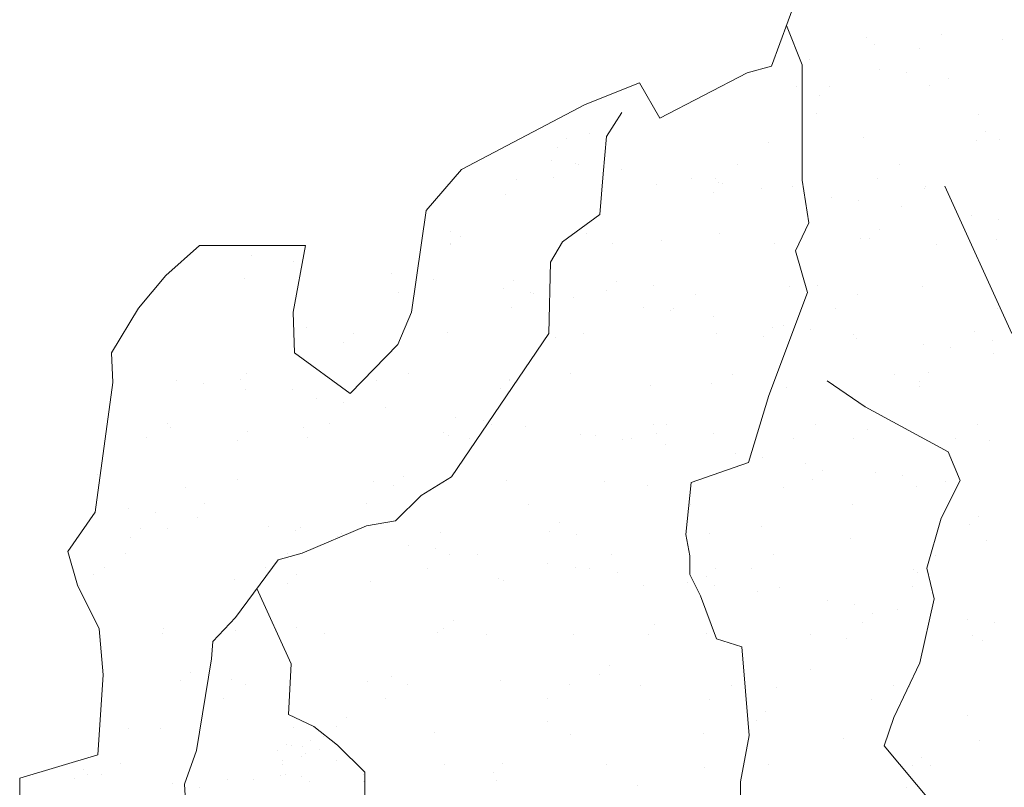
# Model space of a CAD drawing. Units: inches. Extents: x 1986 to 21484, y -1816 to 2016.
# Tile 19 of 85: x 2150.111 to 2157.681, y 1892.429 to 1898.331. Entities that reach past the tile are written whole.
import ezdxf

# ---------------------------------------------------------------- set-up
doc = ezdxf.new("R2010")
doc.units = ezdxf.units.IN
doc.layers.add('L-PLNT', color=84, linetype='Continuous', lineweight=13)

# ---------------------------------------------------------------- blocks, each defined once
blk = doc.blocks.new('PLANT-SHRUB')
for p, q in [((2155.8904, 1897.9733), (2156.12, 1898.5989)), ((2156.1272, 1897.9836), (2156.0052, 1898.2861)), ((2156.6216, 1898.1917), (2156.6216, 1898.1917)), ((2157.1978, 1898.2196), (2157.1978, 1898.2196)), ((2157.6678, 1898.1784), (2157.6678, 1898.1784)), ((2156.6845, 1898.1369), (2156.6845, 1898.1369)), ((2157.0293, 1898.1122), (2157.0293, 1898.1122)), ((2156.1795, 1898.0231), (2156.1795, 1898.0231)), ((2155.7025, 1897.9211), (2155.8904, 1897.9733)), ((2156.1272, 1897.7988), (2156.1272, 1897.9836)), ((2156.7223, 1897.9516), (2156.7223, 1897.9516)), ((2155.0321, 1897.574), (2155.7025, 1897.9211)), ((2156.9304, 1897.9242), (2156.9304, 1897.9242)), ((2157.2553, 1897.8814), (2157.2553, 1897.8814)), ((2154.4581, 1897.6783), (2154.8755, 1897.8452)), ((2154.8755, 1897.8452), (2155.0321, 1897.574)), ((2156.0812, 1897.817), (2156.0812, 1897.817)), ((2156.1275, 1897.0972), (2156.1272, 1897.7988)), ((2156.3368, 1897.8183), (2156.3368, 1897.8183)), ((2157.1035, 1897.8219), (2157.1035, 1897.8219)), ((2156.2632, 1897.7508), (2156.2632, 1897.7508)), ((2153.5085, 1897.1778), (2154.4581, 1897.6783)), ((2154.6228, 1897.4336), (2154.7404, 1897.6164)), ((2154.7404, 1897.6164), (2154.7404, 1897.6164)), ((2156.2372, 1897.6076), (2156.2372, 1897.6076)), ((2157.4818, 1897.6053), (2157.4818, 1897.6053)), ((2154.3162, 1897.4184), (2154.3162, 1897.4184)), ((2154.4945, 1897.4556), (2154.4945, 1897.4556)), ((2154.5967, 1897.1463), (2154.6228, 1897.4336)), ((2156.5964, 1897.4216), (2156.5964, 1897.4216)), ((2157.5383, 1897.4675), (2157.5383, 1897.4675)), ((2157.6426, 1897.4083), (2157.6426, 1897.4083)), ((2154.2425, 1897.3509), (2154.2425, 1897.3509)), ((2155.8654, 1897.3862), (2155.8654, 1897.3862)), ((2157.4646, 1897.4), (2157.4646, 1897.4)), ((2154.2022, 1897.2486), (2154.2022, 1897.2486)), ((2154.3858, 1897.2233), (2154.3858, 1897.2233)), ((2154.4102, 1897.2212), (2154.4102, 1897.2212)), ((2155.6304, 1897.2211), (2155.6304, 1897.2211)), ((2156.875, 1897.2188), (2156.875, 1897.2188)), ((2153.2371, 1896.865), (2153.5085, 1897.1778)), ((2154.2172, 1897.1159), (2154.2172, 1897.1159)), ((2154.5705, 1896.8329), (2154.5967, 1897.1463)), ((2154.7352, 1897.1784), (2154.7352, 1897.1784)), ((2155.278, 1897.1069), (2155.278, 1897.1069)), ((2155.4619, 1897.1137), (2155.4619, 1897.1137)), ((2156.7065, 1897.1114), (2156.7065, 1897.1114)), ((2153.9303, 1897.0992), (2153.9303, 1897.0992)), ((2155.0098, 1897.0603), (2155.0098, 1897.0603)), ((2155.4861, 1897.0795), (2155.4861, 1897.0795)), ((2155.5177, 1897.0676), (2155.5177, 1897.0676)), ((2155.811, 1897.0368), (2155.811, 1897.0368)), ((2156.056, 1897.0469), (2156.056, 1897.0469)), ((2156.1275, 1897.0972), (2156.1275, 1897.0972)), ((2156.1788, 1896.7685), (2156.1275, 1897.0972)), ((2157.0668, 1897.0355), (2157.0668, 1897.0355)), ((2157.0784, 1897.0518), (2157.0784, 1897.0518)), ((2157.224, 1897.0515), (2157.739, 1895.9176)), ((2153.8447, 1896.9864), (2153.8447, 1896.9864)), ((2155.444, 1897.0001), (2155.444, 1897.0001)), ((2156.3538, 1896.9653), (2156.3538, 1896.9653)), ((2156.5619, 1896.9379), (2156.5619, 1896.9379)), ((2156.8868, 1896.8951), (2156.8868, 1896.8951)), ((2153.1223, 1896.0829), (2153.2371, 1896.865)), ((2153.2371, 1896.865), (2153.2371, 1896.865)), ((2154.283, 1896.624), (2154.5705, 1896.8329)), ((2157.4297, 1896.8237), (2157.4297, 1896.8237)), ((2156.0761, 1896.5528), (2156.1788, 1896.7685)), ((2157.6377, 1896.7963), (2157.6377, 1896.7963)), ((2153.4232, 1896.6989), (2153.4232, 1896.6989)), ((2153.497, 1896.6678), (2153.497, 1896.6678)), ((2154.4694, 1896.6855), (2154.4694, 1896.6855)), ((2155.4918, 1896.6904), (2155.4918, 1896.6904)), ((2156.5712, 1896.6515), (2156.5712, 1896.6515)), ((2156.7191, 1896.7168), (2156.7191, 1896.7168)), ((2151.2335, 1896.3644), (2151.4944, 1896.5938)), ((2151.4944, 1896.5938), (2152.3084, 1896.5938)), ((2152.3084, 1896.5938), (2152.2144, 1896.0829)), ((2153.4233, 1896.6003), (2153.4233, 1896.6003)), ((2153.4251, 1896.6113), (2153.4251, 1896.6113)), ((2154.1915, 1896.4672), (2154.283, 1896.624)), ((2154.6697, 1896.609), (2154.6697, 1896.609)), ((2155.0462, 1896.6356), (2155.0462, 1896.6356)), ((2155.9144, 1896.6068), (2155.9144, 1896.6068)), ((2156.6455, 1896.6493), (2156.6455, 1896.6493)), ((2157.159, 1896.6045), (2157.159, 1896.6045)), ((2157.6174, 1896.6382), (2157.6174, 1896.6382)), ((2151.8901, 1896.5182), (2151.8901, 1896.5182)), ((2156.1686, 1896.2344), (2156.0761, 1896.5528)), ((2152.215, 1896.4754), (2152.215, 1896.4754)), ((2154.1785, 1895.9188), (2154.1915, 1896.4672)), ((2151.0248, 1896.1142), (2151.2335, 1896.3644)), ((2152.9659, 1896.3765), (2152.9659, 1896.3765)), ((2151.8366, 1896.3375), (2151.8366, 1896.3375)), ((2153.2908, 1896.3337), (2153.2908, 1896.3337)), ((2153.9052, 1896.3291), (2153.9052, 1896.3291)), ((2154.6985, 1896.317), (2154.6985, 1896.317)), ((2154.9846, 1896.2902), (2154.9846, 1896.2902)), ((2156.0308, 1896.2768), (2156.0308, 1896.2768)), ((2156.2476, 1896.2848), (2156.2476, 1896.2848)), ((2157.0532, 1896.2817), (2157.0532, 1896.2817)), ((2153.0255, 1896.2357), (2153.0255, 1896.2357)), ((2153.8337, 1896.2623), (2153.8337, 1896.2623)), ((2154.0417, 1896.2349), (2154.0417, 1896.2349)), ((2154.063, 1896.2225), (2154.063, 1896.2225)), ((2154.6248, 1896.2495), (2154.6248, 1896.2495)), ((2155.3076, 1896.2202), (2155.3076, 1896.2202)), ((2155.8693, 1895.4412), (2156.1686, 1896.2344)), ((2156.5523, 1896.218), (2156.5523, 1896.218)), ((2154.3667, 1896.1921), (2154.3667, 1896.1921)), ((2150.8161, 1895.7701), (2151.0248, 1896.1142)), ((2152.2144, 1896.0829), (2152.2249, 1895.7701)), ((2153.018, 1895.8326), (2153.1223, 1896.0829)), ((2153.8945, 1896.1151), (2153.8945, 1896.1151)), ((2154.9095, 1896.1206), (2154.9095, 1896.1206)), ((2155.1176, 1896.0933), (2155.1176, 1896.0933)), ((2155.1391, 1896.1129), (2155.1391, 1896.1129)), ((2155.4425, 1896.0505), (2155.4425, 1896.0505)), ((2156.3837, 1896.1106), (2156.3837, 1896.1106)), ((2157.6284, 1896.1083), (2157.6284, 1896.1083)), ((2155.9854, 1895.979), (2155.9854, 1895.979)), ((2152.3185, 1895.9677), (2152.3185, 1895.9677)), ((2152.6778, 1895.9171), (2152.6778, 1895.9171)), ((2153.398, 1895.9288), (2153.398, 1895.9288)), ((2153.4319, 1894.8175), (2154.1785, 1895.9188)), ((2154.1785, 1895.9188), (2154.1785, 1895.9188)), ((2154.4442, 1895.9154), (2154.4442, 1895.9154)), ((2155.4666, 1895.9203), (2155.4666, 1895.9203)), ((2155.8263, 1895.8987), (2155.8263, 1895.8987)), ((2155.8999, 1895.9662), (2155.8999, 1895.9662)), ((2156.1934, 1895.9516), (2156.1934, 1895.9516)), ((2156.5183, 1895.9088), (2156.5183, 1895.9088)), ((2157.4491, 1895.934), (2157.4491, 1895.934)), ((2152.6042, 1895.8496), (2152.6042, 1895.8496)), ((2152.6527, 1895.4572), (2153.018, 1895.8326)), ((2154.227, 1895.885), (2154.227, 1895.885)), ((2156.5461, 1895.8815), (2156.5461, 1895.8815)), ((2157.0612, 1895.8374), (2157.0612, 1895.8374)), ((2157.5922, 1895.8681), (2157.5922, 1895.8681)), ((2150.8265, 1895.5407), (2150.8161, 1895.7701)), ((2152.2249, 1895.7701), (2152.6527, 1895.4572)), ((2157.2692, 1895.81), (2157.2692, 1895.81)), ((2157.5941, 1895.7672), (2157.5941, 1895.7672)), ((2151.8577, 1895.6127), (2151.8577, 1895.6127)), ((2153.1023, 1895.6105), (2153.1023, 1895.6105)), ((2154.347, 1895.6082), (2154.347, 1895.6082)), ((2155.5916, 1895.606), (2155.5916, 1895.606)), ((2156.8362, 1895.6037), (2156.8362, 1895.6037)), ((2157.1014, 1895.6154), (2157.1014, 1895.6154)), ((2150.6908, 1894.5452), (2150.8265, 1895.5407)), ((2151.3136, 1895.5592), (2151.3136, 1895.5592)), ((2151.5216, 1895.5319), (2151.5216, 1895.5319)), ((2151.8114, 1895.5674), (2151.8114, 1895.5674)), ((2152.8576, 1895.5541), (2152.8576, 1895.5541)), ((2153.8793, 1895.5663), (2153.8793, 1895.5663)), ((2153.88, 1895.559), (2153.88, 1895.559)), ((2154.9594, 1895.5201), (2154.9594, 1895.5201)), ((2155.4285, 1895.5342), (2155.4285, 1895.5342)), ((2156.32, 1895.5542), (2156.6117, 1895.3538)), ((2157.0277, 1895.5479), (2157.0277, 1895.5479)), ((2151.8465, 1895.4891), (2151.8465, 1895.4891)), ((2152.2064, 1895.4851), (2152.2064, 1895.4851)), ((2152.6527, 1895.4572), (2152.6527, 1895.4572)), ((2153.8056, 1895.4988), (2153.8056, 1895.4988)), ((2155.7151, 1894.9276), (2155.8693, 1895.4412)), ((2156.0056, 1895.5067), (2156.0056, 1895.5067)), ((2157.028, 1895.5116), (2157.028, 1895.5116)), ((2152.3894, 1895.4176), (2152.3894, 1895.4176)), ((2152.5974, 1895.3902), (2152.5974, 1895.3902)), ((2152.9223, 1895.3474), (2152.9223, 1895.3474)), ((2156.6117, 1895.3538), (2157.2499, 1895.0076)), ((2151.2509, 1895.2262), (2151.2509, 1895.2262)), ((2152.4956, 1895.2239), (2152.4956, 1895.2239)), ((2153.4652, 1895.276), (2153.4652, 1895.276)), ((2153.6732, 1895.2486), (2153.6732, 1895.2486)), ((2153.7402, 1895.2217), (2153.7402, 1895.2217)), ((2154.9848, 1895.2194), (2154.9848, 1895.2194)), ((2155.0808, 1895.2156), (2155.0808, 1895.2156)), ((2156.2295, 1895.2172), (2156.2295, 1895.2172)), ((2157.4741, 1895.2149), (2157.4741, 1895.2149)), ((2151.271, 1895.1927), (2151.271, 1895.1927)), ((2151.8587, 1895.1665), (2151.8587, 1895.1665)), ((2152.2934, 1895.1976), (2152.2934, 1895.1976)), ((2153.3728, 1895.1587), (2153.3728, 1895.1587)), ((2153.9982, 1895.2058), (2153.9982, 1895.2058)), ((2154.419, 1895.1453), (2154.419, 1895.1453)), ((2155.0071, 1895.1481), (2155.0071, 1895.1481)), ((2155.4414, 1895.1502), (2155.4414, 1895.1502)), ((2156.6299, 1895.1834), (2156.6299, 1895.1834)), ((2151.0824, 1895.1188), (2151.0824, 1895.1188)), ((2151.785, 1895.099), (2151.785, 1895.099)), ((2152.327, 1895.1166), (2152.327, 1895.1166)), ((2153.4078, 1895.1343), (2153.4078, 1895.1343)), ((2153.5717, 1895.1143), (2153.5717, 1895.1143)), ((2154.541, 1895.1343), (2154.541, 1895.1343)), ((2154.7491, 1895.107), (2154.7491, 1895.107)), ((2154.8163, 1895.1121), (2154.8163, 1895.1121)), ((2155.074, 1895.0642), (2155.074, 1895.0642)), ((2156.0609, 1895.1098), (2156.0609, 1895.1098)), ((2156.5209, 1895.1114), (2156.5209, 1895.1114)), ((2157.3056, 1895.1075), (2157.3056, 1895.1075)), ((2157.5671, 1895.098), (2157.5671, 1895.098)), ((2155.6169, 1894.9927), (2155.6169, 1894.9927)), ((2157.2499, 1895.0076), (2157.3411, 1894.7889)), ((2155.2731, 1894.7735), (2155.7151, 1894.9276)), ((2155.7151, 1894.9276), (2155.7151, 1894.9276)), ((2155.8249, 1894.9653), (2155.8249, 1894.9653)), ((2156.1498, 1894.9225), (2156.1498, 1894.9225)), ((2150.7068, 1894.8362), (2150.7068, 1894.8362)), ((2156.2822, 1894.8648), (2156.2822, 1894.8648)), ((2156.6927, 1894.8511), (2156.6927, 1894.8511)), ((2151.7862, 1894.7973), (2151.7862, 1894.7973)), ((2152.8324, 1894.784), (2152.8324, 1894.784)), ((2153.0601, 1894.8157), (2153.0601, 1894.8157)), ((2153.1967, 1894.6738), (2153.4319, 1894.8175)), ((2153.4319, 1894.8175), (2153.4319, 1894.8175)), ((2153.8548, 1894.7889), (2153.8548, 1894.7889)), ((2154.6093, 1894.7835), (2154.6093, 1894.7835)), ((2155.232, 1894.373), (2155.2731, 1894.7735)), ((2156.2086, 1894.7973), (2156.2086, 1894.7973)), ((2156.9007, 1894.8237), (2156.9007, 1894.8237)), ((2157.3411, 1894.7889), (2157.1952, 1894.4974)), ((2157.2256, 1894.7809), (2157.2256, 1894.7809)), ((2151.3872, 1894.7345), (2151.3872, 1894.7345)), ((2152.9865, 1894.7482), (2152.9865, 1894.7482)), ((2154.9343, 1894.75), (2154.9343, 1894.75)), ((2155.9804, 1894.7366), (2155.9804, 1894.7366)), ((2157.0028, 1894.7415), (2157.0028, 1894.7415)), ((2151.5349, 1894.6119), (2151.5349, 1894.6119)), ((2152.7795, 1894.6097), (2152.7795, 1894.6097)), ((2153.0006, 1894.478), (2153.1967, 1894.6738)), ((2154.0242, 1894.6074), (2154.0242, 1894.6074)), ((2150.482, 1894.2428), (2150.6908, 1894.5452)), ((2150.9451, 1894.573), (2150.9451, 1894.573)), ((2151.1531, 1894.5456), (2151.1531, 1894.5456)), ((2155.2688, 1894.6051), (2155.2688, 1894.6051)), ((2156.5134, 1894.6029), (2156.5134, 1894.6029)), ((2151.478, 1894.5028), (2151.478, 1894.5028)), ((2152.7784, 1894.4388), (2153.0006, 1894.478)), ((2154.2616, 1894.4649), (2154.2616, 1894.4649)), ((2157.1952, 1894.4974), (2157.0858, 1894.1148)), ((2157.4837, 1894.514), (2157.4837, 1894.514)), ((2151.0395, 1894.4158), (2151.0395, 1894.4158)), ((2151.2458, 1894.4226), (2151.2458, 1894.4226)), ((2152.0209, 1894.4313), (2152.0209, 1894.4313)), ((2152.2289, 1894.4039), (2152.2289, 1894.4039)), ((2152.2682, 1894.4275), (2152.2682, 1894.4275)), ((2152.2818, 1894.2298), (2152.7784, 1894.4388)), ((2152.5887, 1894.3837), (2152.5887, 1894.3837)), ((2153.3477, 1894.3886), (2153.3477, 1894.3886)), ((2154.1879, 1894.3974), (2154.1879, 1894.3974)), ((2155.4162, 1894.3802), (2155.4162, 1894.3802)), ((2155.8108, 1894.4328), (2155.8108, 1894.4328)), ((2157.41, 1894.4465), (2157.41, 1894.4465)), ((2150.9658, 1894.3483), (2150.9658, 1894.3483)), ((2152.5538, 1894.3612), (2152.5538, 1894.3612)), ((2154.3938, 1894.3752), (2154.3938, 1894.3752)), ((2155.2628, 1894.2086), (2155.232, 1894.373)), ((2156.4957, 1894.3413), (2156.4957, 1894.3413)), ((2157.5419, 1894.3279), (2157.5419, 1894.3279)), ((2150.5551, 1893.9822), (2150.482, 1894.2428)), ((2152.0988, 1894.1776), (2152.2818, 1894.2298)), ((2153.0967, 1894.2897), (2153.0967, 1894.2897)), ((2153.3047, 1894.2623), (2153.3047, 1894.2623)), ((2150.9282, 1894.2254), (2150.9282, 1894.2254)), ((2151.7707, 1893.7361), (2152.0988, 1894.1776)), ((2152.1728, 1894.2231), (2152.1728, 1894.2231)), ((2153.4174, 1894.2209), (2153.4174, 1894.2209)), ((2153.6297, 1894.2195), (2153.6297, 1894.2195)), ((2154.6621, 1894.2186), (2154.6621, 1894.2186)), ((2155.2628, 1894.0648), (2155.2628, 1894.2086)), ((2155.9067, 1894.2163), (2155.9067, 1894.2163)), ((2157.1513, 1894.2141), (2157.1513, 1894.2141)), ((2150.7596, 1894.118), (2150.7596, 1894.118)), ((2152.0043, 1894.1158), (2152.0043, 1894.1158)), ((2153.2489, 1894.1135), (2153.2489, 1894.1135)), ((2154.1725, 1894.148), (2154.1725, 1894.148)), ((2154.3806, 1894.1207), (2154.3806, 1894.1207)), ((2154.4935, 1894.1112), (2154.4935, 1894.1112)), ((2154.7055, 1894.0779), (2154.7055, 1894.0779)), ((2155.463, 1894.1141), (2155.463, 1894.1141)), ((2155.7382, 1894.109), (2155.7382, 1894.109)), ((2156.9828, 1894.1067), (2156.9828, 1894.1067)), ((2157.0122, 1894.082), (2157.0122, 1894.082)), ((2157.0858, 1894.1148), (2157.1405, 1893.878)), ((2150.6816, 1894.0661), (2150.6816, 1894.0661)), ((2151.7611, 1894.0272), (2151.7611, 1894.0272)), ((2152.2409, 1894.0651), (2152.2409, 1894.0651)), ((2152.8072, 1894.0139), (2152.8072, 1894.0139)), ((2153.7901, 1894.0329), (2153.7901, 1894.0329)), ((2153.8296, 1894.0188), (2153.8296, 1894.0188)), ((2155.2484, 1894.0064), (2155.2484, 1894.0064)), ((2155.3451, 1893.9005), (2155.2628, 1894.0648)), ((2155.3894, 1894.0466), (2155.3894, 1894.0466)), ((2150.7221, 1893.6485), (2150.5551, 1893.9822)), ((2150.568, 1893.9838), (2150.568, 1893.9838)), ((2151.9348, 1893.9568), (2152.1979, 1893.3779)), ((2152.1673, 1893.9976), (2152.1673, 1893.9976)), ((2154.9091, 1893.9799), (2154.9091, 1893.9799)), ((2155.4564, 1893.979), (2155.4564, 1893.979)), ((2155.7813, 1893.9362), (2155.7813, 1893.9362)), ((2155.9553, 1893.9665), (2155.9553, 1893.9665)), ((2156.9777, 1893.9714), (2156.9777, 1893.9714)), ((2155.4684, 1893.5718), (2155.3451, 1893.9005)), ((2156.3242, 1893.8648), (2156.3242, 1893.8648)), ((2157.1405, 1893.878), (2157.0311, 1893.386)), ((2156.5322, 1893.8374), (2156.5322, 1893.8374)), ((2156.8571, 1893.7946), (2156.8571, 1893.7946)), ((2151.5949, 1893.5501), (2151.7707, 1893.7361)), ((2153.4424, 1893.7143), (2153.4424, 1893.7143)), ((2156.6645, 1893.7634), (2156.6645, 1893.7634)), ((2157.4, 1893.7231), (2157.4, 1893.7231)), ((2150.7534, 1893.2939), (2150.7221, 1893.6485)), ((2151.2206, 1893.6525), (2151.2206, 1893.6525)), ((2151.7695, 1893.633), (2151.7695, 1893.633)), ((2152.243, 1893.6574), (2152.243, 1893.6574)), ((2153.3687, 1893.6468), (2153.3687, 1893.6468)), ((2154.9916, 1893.6821), (2154.9916, 1893.6821)), ((2156.5908, 1893.6959), (2156.5908, 1893.6959)), ((2157.608, 1893.6958), (2157.608, 1893.6958)), ((2151.2121, 1893.6111), (2151.2121, 1893.6111)), ((2151.5846, 1893.4158), (2151.5949, 1893.5501)), ((2152.4567, 1893.6089), (2152.4567, 1893.6089)), ((2153.3225, 1893.6185), (2153.3225, 1893.6185)), ((2153.7014, 1893.6066), (2153.7014, 1893.6066)), ((2154.3687, 1893.6052), (2154.3687, 1893.6052)), ((2154.946, 1893.6043), (2154.946, 1893.6043)), ((2155.3911, 1893.6101), (2155.3911, 1893.6101)), ((2155.4684, 1893.5718), (2155.4684, 1893.5718)), ((2155.6637, 1893.5102), (2155.4684, 1893.5718)), ((2156.1906, 1893.6021), (2156.1906, 1893.6021)), ((2156.4705, 1893.5712), (2156.4705, 1893.5712)), ((2157.4353, 1893.5998), (2157.4353, 1893.5998)), ((2157.5167, 1893.5578), (2157.5167, 1893.5578)), ((2155.7187, 1892.8278), (2155.6637, 1893.5102)), ((2151.4708, 1892.7131), (2151.5846, 1893.4158)), ((2152.1979, 1893.3779), (2152.1786, 1892.9883)), ((2154.6439, 1893.3635), (2154.6439, 1893.3635)), ((2156.193, 1893.3313), (2156.193, 1893.3313)), ((2157.0311, 1893.386), (2156.8305, 1892.967)), ((2150.7124, 1892.6794), (2150.7534, 1893.2939)), ((2151.3481, 1893.2469), (2151.3481, 1893.2469)), ((2151.4218, 1893.3144), (2151.4218, 1893.3144)), ((2151.7359, 1893.2571), (2151.7359, 1893.2571)), ((2152.9709, 1893.2823), (2152.9709, 1893.2823)), ((2153.8045, 1893.2487), (2153.8045, 1893.2487)), ((2154.5702, 1893.296), (2154.5702, 1893.296)), ((2151.85, 1893.2223), (2151.85, 1893.2223)), ((2152.7821, 1893.2438), (2152.7821, 1893.2438)), ((2153.0946, 1893.2201), (2153.0946, 1893.2201)), ((2154.3393, 1893.2178), (2154.3393, 1893.2178)), ((2154.8839, 1893.2098), (2154.8839, 1893.2098)), ((2155.5839, 1893.2155), (2155.5839, 1893.2155)), ((2155.9301, 1893.1964), (2155.9301, 1893.1964)), ((2156.8285, 1893.2133), (2156.8285, 1893.2133)), ((2156.9525, 1893.2013), (2156.9525, 1893.2013)), ((2151.6815, 1893.1149), (2151.6815, 1893.1149)), ((2152.9261, 1893.1127), (2152.9261, 1893.1127)), ((2154.1707, 1893.1104), (2154.1707, 1893.1104)), ((2155.4154, 1893.1082), (2155.4154, 1893.1082)), ((2156.66, 1893.1059), (2156.66, 1893.1059)), ((2152.1786, 1892.9883), (2152.3724, 1892.8961)), ((2152.6232, 1892.9636), (2152.6232, 1892.9636)), ((2155.7717, 1892.9452), (2155.7717, 1892.9452)), ((2155.8453, 1893.0127), (2155.8453, 1893.0127)), ((2156.8305, 1892.967), (2156.7576, 1892.7483)), ((2157.3945, 1892.9806), (2157.3945, 1892.9806)), ((2150.9503, 1892.8824), (2150.9503, 1892.8824)), ((2151.1954, 1892.8824), (2151.1954, 1892.8824)), ((2152.2178, 1892.8873), (2152.2178, 1892.8873)), ((2152.2178, 1892.8873), (2152.2178, 1892.8873)), ((2152.3724, 1892.8961), (2152.5548, 1892.7529)), ((2152.5496, 1892.8961), (2152.5496, 1892.8961)), ((2154.1724, 1892.9315), (2154.1724, 1892.9315)), ((2152.4451, 1892.8205), (2152.4451, 1892.8205)), ((2153.2973, 1892.8484), (2153.2973, 1892.8484)), ((2154.3435, 1892.8351), (2154.3435, 1892.8351)), ((2155.3659, 1892.84), (2155.3659, 1892.84)), ((2155.6536, 1892.4702), (2155.7187, 1892.8278)), ((2156.4454, 1892.8011), (2156.4454, 1892.8011)), ((2152.1637, 1892.7571), (2152.1637, 1892.7571)), ((2152.2016, 1892.7518), (2152.2016, 1892.7518)), ((2152.2848, 1892.7409), (2152.2848, 1892.7409)), ((2152.3504, 1892.7856), (2152.3504, 1892.7856)), ((2152.4148, 1892.7238), (2152.4148, 1892.7238)), ((2152.5548, 1892.7529), (2152.7633, 1892.5446)), ((2156.7576, 1892.7483), (2157.1223, 1892.3111)), ((2157.4915, 1892.7877), (2157.4915, 1892.7877)), ((2150.1112, 1892.4992), (2150.7124, 1892.6794)), ((2151.3777, 1892.4547), (2151.4708, 1892.7131)), ((2152.0962, 1892.7142), (2152.0962, 1892.7142)), ((2152.2766, 1892.666), (2152.2766, 1892.666)), ((2152.306, 1892.693), (2152.306, 1892.693)), ((2152.5941, 1892.7133), (2152.5941, 1892.7133)), ((2157.0468, 1892.6619), (2157.0468, 1892.6619)), ((2150.6026, 1892.5638), (2150.6026, 1892.5638)), ((2150.8893, 1892.6103), (2150.8893, 1892.6103)), ((2152.134, 1892.608), (2152.134, 1892.608)), ((2152.134, 1892.608), (2152.134, 1892.608)), ((2152.1342, 1892.6357), (2152.1342, 1892.6357)), ((2152.5432, 1892.6377), (2152.5432, 1892.6377)), ((2153.3786, 1892.6058), (2153.3786, 1892.6058)), ((2153.8247, 1892.6129), (2153.8247, 1892.6129)), ((2154.6232, 1892.6035), (2154.6232, 1892.6035)), ((2155.3739, 1892.5807), (2155.3739, 1892.5807)), ((2155.8679, 1892.6013), (2155.8679, 1892.6013)), ((2156.9731, 1892.5944), (2156.9731, 1892.5944)), ((2157.1125, 1892.599), (2157.1125, 1892.599)), ((2150.1112, 1892.0787), (2150.1112, 1892.4992)), ((2150.5289, 1892.4963), (2150.5289, 1892.4963)), ((2150.6312, 1892.5259), (2150.6312, 1892.5259)), ((2150.741, 1892.5302), (2150.741, 1892.5302)), ((2151.9085, 1892.4931), (2151.9085, 1892.4931)), ((2152.1174, 1892.5202), (2152.1174, 1892.5202)), ((2152.1518, 1892.5316), (2152.1518, 1892.5316)), ((2152.1518, 1892.5316), (2152.1518, 1892.5316)), ((2152.2772, 1892.5114), (2152.2772, 1892.5114)), ((2152.7571, 1892.5257), (2152.7571, 1892.5257)), ((2152.7633, 1892.5446), (2152.7633, 1892.2842)), ((2153.751, 1892.5454), (2153.751, 1892.5454)), ((2151.2839, 1892.4587), (2151.2839, 1892.4587)), ((2151.3881, 1892.279), (2151.3777, 1892.4547)), ((2151.4919, 1892.4313), (2151.4919, 1892.4313)), ((2151.7107, 1892.487), (2151.7107, 1892.487)), ((2152.3403, 1892.4776), (2152.3403, 1892.4776)), ((2152.7569, 1892.4737), (2152.7569, 1892.4737)), ((2152.7569, 1892.4737), (2152.7569, 1892.4737)), ((2152.7588, 1892.4722), (2152.7588, 1892.4722)), ((2153.7793, 1892.4786), (2153.7793, 1892.4786)), ((2154.8587, 1892.4397), (2154.8587, 1892.4397)), ((2155.6536, 1892.2751), (2155.6536, 1892.4702)), ((2156.9273, 1892.4312), (2156.9273, 1892.4312))]:
    blk.add_line(p, q)

msp = doc.modelspace()

# ---------------------------------------------------------------- block references
at = {"layer": 'L-PLNT'}
msp.add_blockref('PLANT-SHRUB', (0, 0), dxfattribs=at)

doc.saveas('drawing.dxf')
